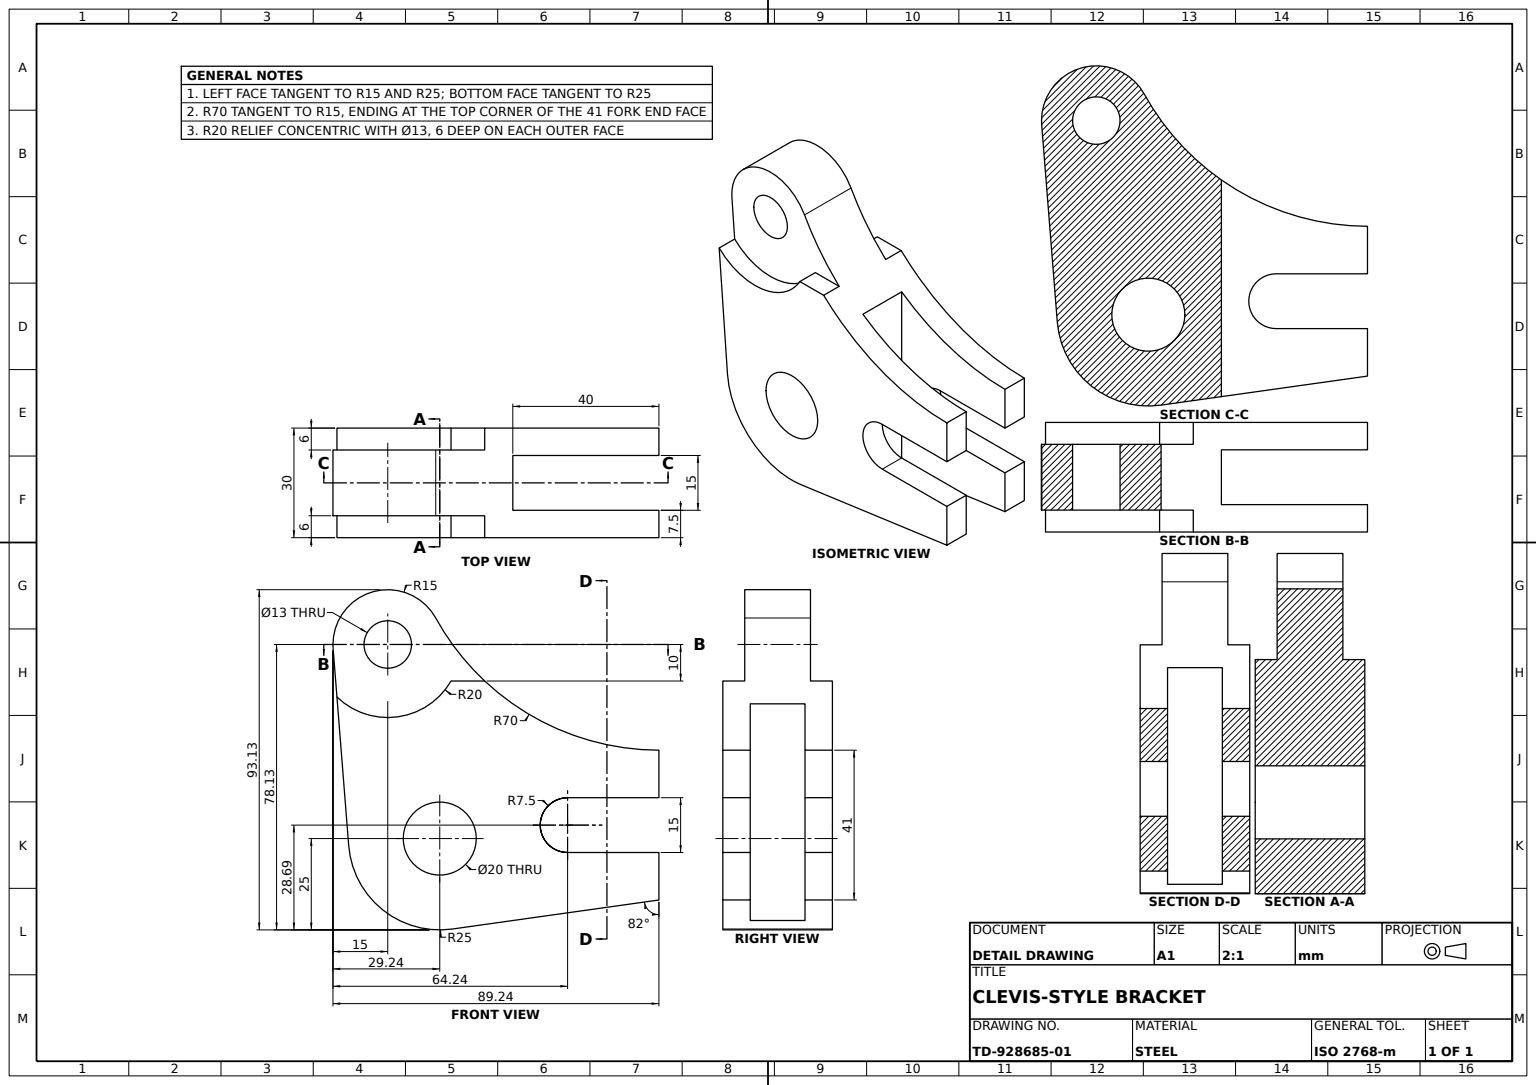
from build123d import *

# Parameters (mm, degrees)
BRACKET_PROFILE_SKETCH_R       = 10
BRACKET_PROFILE_SKETCH_R_2     = 6.5
BRACKET_BODY_30_THICK_DEPTH    = 15
SIDE_STEP_CUT_20X10X6_DEPTH    = 6
FORKED_SLOT_15_WIDE_DEPTH      = 93.011635333
FORKED_SLOT_15_WIDE_DEPTH_BACK = 93.011635333
FORK_SLOT_SKETCH_W             = 15
FORK_SLOT_SKETCH_H             = 40


with BuildPart() as part:
    # Bracket Profile Sketch → Bracket Body 30 Thick (new, symmetric)
    with BuildSketch(Plane(origin=(0, 0, 0), x_dir=(0, 0, -1), z_dir=(1, 0, 0))):
        with BuildLine():
            Line((-24.92209858, -1.972055368), (-29.188306629, 51.942687225))
            ThreePointArc((-29.188306629, 51.942687225), (-18.546726282, 67.492876488), (-1.101285774, 60.371905777))
            ThreePointArc((-1.101285774, 60.371905777), (24.520233718, 33.956144929), (60, 24.186760769))
            Line((60, 24.186760769), (60, 11.186760769))
            Line((60, 11.186760769), (35, 11.186760769))
            ThreePointArc((35, 11.186760769), (27.5, 3.686760769), (35, -3.813239231))
            Line((35, -3.813239231), (60, -3.813239231))
            Line((60, -3.813239231), (60, -16.813239231))
            Line((60, -16.813239231), (3.479327524, -24.756701719))
            ThreePointArc((3.479327524, -24.756701719), (-15.643948829, -19.500432432), (-24.92209858, -1.972055368))
        make_face()
        Circle(BRACKET_PROFILE_SKETCH_R, mode=Mode.SUBTRACT)
        with Locations((-14.235047481, 53.125920446)):
            Circle(BRACKET_PROFILE_SKETCH_R_2, mode=Mode.SUBTRACT)
    extrude(amount=BRACKET_BODY_30_THICK_DEPTH, both=True)

    # Side Step Sketch → Side Step Cut 20x10x6 (cut)
    with BuildSketch(Plane(origin=(15, 0, 0), x_dir=(0, 0, -1), z_dir=(1, 0, 0))):
        with BuildLine():
            Line((3.085460595, 43.125920446), (12.306235476, 43.125920446))
            ThreePointArc((12.306235476, 43.125920446), (4.925595155, 51.222687515), (-1.101285774, 60.371905777))
            ThreePointArc((-1.101285774, 60.371905777), (-18.546726282, 67.492876488), (-29.188306629, 51.942687225))
            Line((-29.188306629, 51.942687225), (-28.144793013, 38.755152227))
            ThreePointArc((-28.144793013, 38.755152227), (-11.463003291, 33.318957756), (3.085460595, 43.125920446))
        make_face()
    side_step_cut_20x10x6 = extrude(amount=-SIDE_STEP_CUT_20X10X6_DEPTH, mode=Mode.SUBTRACT)

    # Side Step Cut Mirror: Side Step Cut 20x10x6 across plane
    add(side_step_cut_20x10x6.mirror(Plane(origin=(0, 0, 0), x_dir=(0, 0, 1), z_dir=(1, 0, 0))), mode=Mode.SUBTRACT)

    # Fork Slot Sketch → Forked Slot 15 Wide (cut, two sides: drawn at the far end of the back side and taken through both)
    with BuildSketch(Plane(origin=(0, 0, 0), x_dir=(1, 0, 0), z_dir=(0, 1, 0)).offset(-FORKED_SLOT_15_WIDE_DEPTH_BACK)):
        with Locations((0, 40)):
            Rectangle(FORK_SLOT_SKETCH_W, FORK_SLOT_SKETCH_H)
    extrude(amount=FORKED_SLOT_15_WIDE_DEPTH + FORKED_SLOT_15_WIDE_DEPTH_BACK, mode=Mode.SUBTRACT)


solid = part.part
